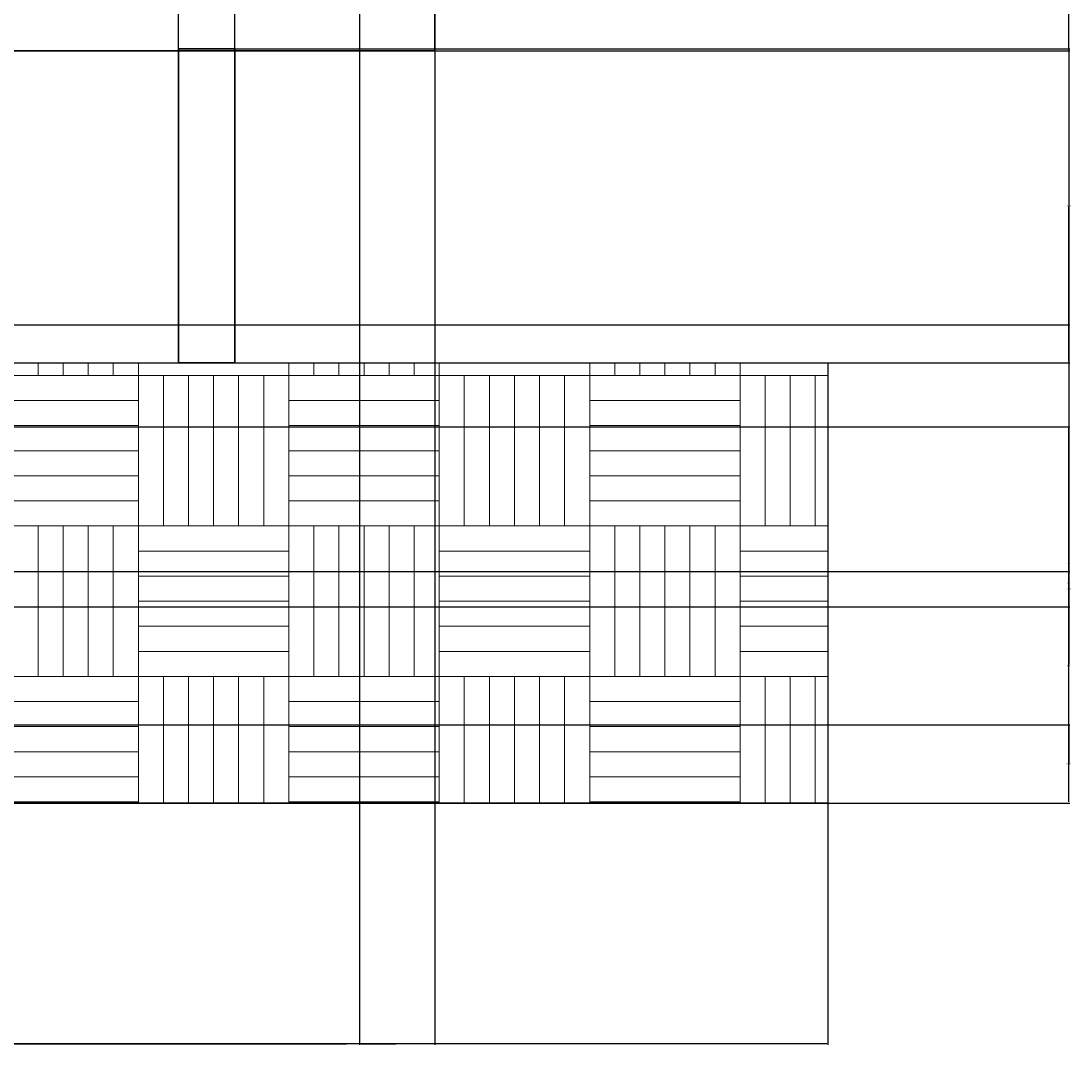
# Model space of a CAD drawing. Units: inches. Extents: x -15 to 605, y -220 to 570.
# Tile 5 of 10: x 438 to 605, y -155 to 9. Entities that reach past the tile are written whole.
import ezdxf

# ---------------------------------------------------------------- set-up
doc = ezdxf.new("R2010")
doc.units = ezdxf.units.IN
doc.header["$MEASUREMENT"] = 0
for name, color, linetype, lineweight in [('A-ANNO-DIMS', 2, 'Continuous', 18), ('A-COLS', 7, 'Continuous', 35), ('A-ELEV', 7, 'Continuous', 35), ('A-ELEV-PATT', 8, 'Continuous', 13), ('C-SITE', 3, 'Continuous', 25)]:
    doc.layers.add(name, color=color, linetype=linetype, lineweight=lineweight)
doc.styles.get("Standard").update_dxf_attribs({"font": 'arial.ttf'})
doc.dimstyles.get("Standard").update_dxf_attribs({"dimtxt": 0.18, "dimasz": 0.18, "dimexe": 0.18, "dimexo": 0.0625, "dimgap": 0.09, "dimtad": 0, "dimtih": 1, "dimtoh": 1, "dimdec": 4, "dimzin": 0, "dimdsep": 46, "dimtxsty": 'Standard', "dimcen": 0.09, "dimadec": 0, "dimazin": 0, "dimtfac": 1, "dimtdec": 4, "dimtofl": 0, "dimtmove": 0, "dimatfit": 3, "dimfxl": 1, "dimtolj": 1, "dimtzin": 0, "dimarcsym": 0})

# ---------------------------------------------------------------- blocks, each defined once
blk = doc.blocks.new('*D7')
at = {"layer": 'A-ANNO-DIMS', "color": 0, "lineweight": -2, "transparency": 16777216}
for p, q in [((23.99, 3.76), (23.99, -154.76)), ((566.72, -116.24), (566.72, -154.76)), ((24.17, -154.58), (294.96, -154.58)), ((566.54, -154.58), (295.75, -154.58))]:
    blk.add_line(p, q, dxfattribs=at)
at = {"layer": 'A-ANNO-DIMS', "color": 0, "transparency": 16777216}
for points in [[(24.17, -154.55), (24.17, -154.61), (23.99, -154.58)], [(566.54, -154.55), (566.54, -154.61), (566.72, -154.58)]]:
    blk.add_solid(points, dxfattribs=at)
at = {"layer": 'Defpoints', "color": 0, "transparency": 16777216}
for p in [(23.99, 3.82), (566.72, -116.18), (566.72, -154.58)]:
    blk.add_point(p, dxfattribs=at)
at = {"layer": 'A-ANNO-DIMS', "color": 0, "transparency": 16777216, "insert": (295.35, -154.58), "char_height": 0.18, "attachment_point": 5}
blk.add_mtext('\\A1;542.7', dxfattribs=at)
blk = doc.blocks.new('*D8')
at = {"layer": 'A-ANNO-DIMS', "color": 0, "lineweight": -2, "transparency": 16777216}
for p, q in [((23.99, 3.88), (23.99, 570.4)), ((24.17, 570.22), (263.7, 570.22)), ((503.81, 570.22), (264.28, 570.22)), ((503.99, 531.88), (503.99, 570.4))]:
    blk.add_line(p, q, dxfattribs=at)
at = {"layer": 'A-ANNO-DIMS', "color": 0, "transparency": 16777216}
for points in [[(24.17, 570.25), (24.17, 570.19), (23.99, 570.22)], [(503.81, 570.25), (503.81, 570.19), (503.99, 570.22)]]:
    blk.add_solid(points, dxfattribs=at)
at = {"layer": 'Defpoints', "color": 0, "transparency": 16777216}
for p in [(503.99, 570.22), (503.99, 531.82), (23.99, 3.82)]:
    blk.add_point(p, dxfattribs=at)
at = {"layer": 'A-ANNO-DIMS', "color": 0, "transparency": 16777216, "insert": (263.99, 570.22), "char_height": 0.18, "attachment_point": 5}
blk.add_mtext('\\A1;480', dxfattribs=at)
blk = doc.blocks.new('*D9')
at = {"layer": 'A-ANNO-DIMS', "color": 0, "lineweight": -2, "transparency": 16777216}
for p, q in [((503.92, 531.82), (-14.59, 531.82)), ((-14.41, 531.64), (-14.41, 208)), ((-14.41, -116), (-14.41, 207.64)), ((23.92, -116.18), (-14.59, -116.18))]:
    blk.add_line(p, q, dxfattribs=at)
at = {"layer": 'A-ANNO-DIMS', "color": 0, "transparency": 16777216}
for points in [[(-14.44, 531.64), (-14.38, 531.64), (-14.41, 531.82)], [(-14.44, -116), (-14.38, -116), (-14.41, -116.18)]]:
    blk.add_solid(points, dxfattribs=at)
at = {"layer": 'Defpoints', "color": 0, "transparency": 16777216}
for p in [(-14.41, 531.82), (503.99, 531.82), (23.99, -116.18)]:
    blk.add_point(p, dxfattribs=at)
at = {"layer": 'A-ANNO-DIMS', "color": 0, "transparency": 16777216, "insert": (-14.41, 207.82), "char_height": 0.18, "attachment_point": 5}
blk.add_mtext('\\A1;648', dxfattribs=at)
blk = doc.blocks.new('*D10')
at = {"layer": 'A-ANNO-DIMS', "color": 0, "lineweight": -2, "transparency": 16777216}
for p, q in [((504.05, 3.82), (605.3, 3.82)), ((605.12, 3.64), (605.12, -56)), ((605.12, -116), (605.12, -56.36)), ((566.78, -116.18), (605.3, -116.18))]:
    blk.add_line(p, q, dxfattribs=at)
at = {"layer": 'A-ANNO-DIMS', "color": 0, "transparency": 16777216}
for points in [[(605.09, 3.64), (605.15, 3.64), (605.12, 3.82)], [(605.09, -116), (605.15, -116), (605.12, -116.18)]]:
    blk.add_solid(points, dxfattribs=at)
at = {"layer": 'Defpoints', "color": 0, "transparency": 16777216}
for p in [(503.99, 3.82), (605.12, 3.82), (566.72, -116.18)]:
    blk.add_point(p, dxfattribs=at)
at = {"layer": 'A-ANNO-DIMS', "color": 0, "transparency": 16777216, "insert": (605.12, -56.18), "char_height": 0.18, "attachment_point": 5}
blk.add_mtext('\\A1;120', dxfattribs=at)
blk = doc.blocks.new('*D11')
at = {"layer": 'A-ANNO-DIMS', "color": 0, "lineweight": -2, "transparency": 16777216}
for p, q in [((492.05, 15.82), (605.3, 15.82)), ((605.12, 15.64), (605.12, 10)), ((605.12, 4), (605.12, 9.64)), ((504.05, 3.82), (605.3, 3.82))]:
    blk.add_line(p, q, dxfattribs=at)
at = {"layer": 'A-ANNO-DIMS', "color": 0, "transparency": 16777216}
for points in [[(605.09, 15.64), (605.15, 15.64), (605.12, 15.82)], [(605.09, 4), (605.15, 4), (605.12, 3.82)]]:
    blk.add_solid(points, dxfattribs=at)
at = {"layer": 'Defpoints', "color": 0, "transparency": 16777216}
for p in [(491.99, 15.82), (605.12, 15.82), (503.99, 3.82)]:
    blk.add_point(p, dxfattribs=at)
at = {"layer": 'A-ANNO-DIMS', "color": 0, "transparency": 16777216, "insert": (605.12, 9.82), "char_height": 0.18, "attachment_point": 5}
blk.add_mtext('\\A1;12', dxfattribs=at)
blk = doc.blocks.new('*D22')
at = {"layer": 'A-ANNO-DIMS', "color": 0, "lineweight": -2, "transparency": 16777216}
for p, q in [((472.17, 4.14), (605.3, 4.14)), ((605.12, 3.96), (605.12, -20.72)), ((605.12, -45.76), (605.12, -21.08)), ((472.17, -45.94), (605.3, -45.94))]:
    blk.add_line(p, q, dxfattribs=at)
at = {"layer": 'A-ANNO-DIMS', "color": 0, "transparency": 16777216}
for points in [[(605.09, 3.96), (605.15, 3.96), (605.12, 4.14)], [(605.09, -45.76), (605.15, -45.76), (605.12, -45.94)]]:
    blk.add_solid(points, dxfattribs=at)
at = {"layer": 'Defpoints', "color": 0, "transparency": 16777216}
for p in [(472.1, 4.14), (605.12, 4.14), (472.1, -45.94)]:
    blk.add_point(p, dxfattribs=at)
at = {"layer": 'A-ANNO-DIMS', "color": 0, "transparency": 16777216, "insert": (605.12, -20.9), "char_height": 0.18, "attachment_point": 5}
blk.add_mtext('\\A1;50.07', dxfattribs=at)
blk = doc.blocks.new('*D31')
at = {"layer": 'A-ANNO-DIMS', "color": 0, "lineweight": -2, "transparency": 16777216}
for p, q in [((382.03, 34.31), (382.03, -154.76)), ((491.99, 15.76), (491.99, -154.76)), ((382.21, -154.58), (436.55, -154.58)), ((491.81, -154.58), (437.46, -154.58))]:
    blk.add_line(p, q, dxfattribs=at)
at = {"layer": 'A-ANNO-DIMS', "color": 0, "transparency": 16777216}
for points in [[(382.21, -154.55), (382.21, -154.61), (382.03, -154.58)], [(491.81, -154.55), (491.81, -154.61), (491.99, -154.58)]]:
    blk.add_solid(points, dxfattribs=at)
at = {"layer": 'Defpoints', "color": 0, "transparency": 16777216}
for p in [(382.03, 34.38), (491.99, 15.82), (491.99, -154.58)]:
    blk.add_point(p, dxfattribs=at)
at = {"layer": 'A-ANNO-DIMS', "color": 0, "transparency": 16777216, "insert": (437.01, -154.58), "char_height": 0.18, "attachment_point": 5}
blk.add_mtext('\\A1;109.96', dxfattribs=at)
blk = doc.blocks.new('*D32')
at = {"layer": 'A-ANNO-DIMS', "color": 0, "lineweight": -2, "transparency": 16777216}
for p, q in [((491.99, 15.76), (491.99, -154.76)), ((503.99, 3.76), (503.99, -154.76)), ((492.17, -154.58), (497.78, -154.58)), ((503.81, -154.58), (498.2, -154.58))]:
    blk.add_line(p, q, dxfattribs=at)
at = {"layer": 'A-ANNO-DIMS', "color": 0, "transparency": 16777216}
for points in [[(492.17, -154.55), (492.17, -154.61), (491.99, -154.58)], [(503.81, -154.55), (503.81, -154.61), (503.99, -154.58)]]:
    blk.add_solid(points, dxfattribs=at)
at = {"layer": 'Defpoints', "color": 0, "transparency": 16777216}
for p in [(491.99, 15.82), (503.99, 3.82), (503.99, -154.58)]:
    blk.add_point(p, dxfattribs=at)
at = {"layer": 'A-ANNO-DIMS', "color": 0, "transparency": 16777216, "insert": (497.99, -154.58), "char_height": 0.18, "attachment_point": 5}
blk.add_mtext('\\A1;12', dxfattribs=at)
blk = doc.blocks.new('*D51')
at = {"layer": 'A-ANNO-DIMS', "color": 0, "lineweight": -2, "transparency": 16777216}
for p, q in [((414, -116.24), (414, -154.76)), ((566.72, -116.24), (566.72, -154.76)), ((414.18, -154.58), (489.9, -154.58)), ((566.54, -154.58), (490.81, -154.58))]:
    blk.add_line(p, q, dxfattribs=at)
at = {"layer": 'A-ANNO-DIMS', "color": 0, "transparency": 16777216}
for points in [[(414.18, -154.55), (414.18, -154.61), (414, -154.58)], [(566.54, -154.55), (566.54, -154.61), (566.72, -154.58)]]:
    blk.add_solid(points, dxfattribs=at)
at = {"layer": 'Defpoints', "color": 0, "transparency": 16777216}
for p in [(414, -116.18), (566.72, -116.18), (566.72, -154.58)]:
    blk.add_point(p, dxfattribs=at)
at = {"layer": 'A-ANNO-DIMS', "color": 0, "transparency": 16777216, "insert": (490.36, -154.58), "char_height": 0.18, "attachment_point": 5}
blk.add_mtext('\\A1;152.72', dxfattribs=at)
blk = doc.blocks.new('*D58')
at = {"layer": 'A-ANNO-DIMS', "color": 0, "lineweight": -2, "transparency": 16777216}
for p, q in [((376.71, -44.82), (376.71, 570.4)), ((376.89, 570.22), (419.58, 570.22)), ((462.92, 570.22), (420.23, 570.22)), ((463.1, -45.87), (463.1, 570.4))]:
    blk.add_line(p, q, dxfattribs=at)
at = {"layer": 'A-ANNO-DIMS', "color": 0, "transparency": 16777216}
for points in [[(376.89, 570.25), (376.89, 570.19), (376.71, 570.22)], [(462.92, 570.25), (462.92, 570.19), (463.1, 570.22)]]:
    blk.add_solid(points, dxfattribs=at)
at = {"layer": 'Defpoints', "color": 0, "transparency": 16777216}
for p in [(463.1, 570.22), (376.71, -44.88), (463.1, -45.94)]:
    blk.add_point(p, dxfattribs=at)
at = {"layer": 'A-ANNO-DIMS', "color": 0, "transparency": 16777216, "insert": (419.9, 570.22), "char_height": 0.18, "attachment_point": 5}
blk.add_mtext('\\A1;86.4', dxfattribs=at)
blk = doc.blocks.new('*D59')
at = {"layer": 'A-ANNO-DIMS', "color": 0, "lineweight": -2, "transparency": 16777216}
for p, q in [((463.1, -45.87), (463.1, 570.4)), ((463.28, 570.22), (467.45, 570.22)), ((471.92, 570.22), (467.75, 570.22)), ((472.1, -45.87), (472.1, 570.4))]:
    blk.add_line(p, q, dxfattribs=at)
at = {"layer": 'A-ANNO-DIMS', "color": 0, "transparency": 16777216}
for points in [[(463.28, 570.25), (463.28, 570.19), (463.1, 570.22)], [(471.92, 570.25), (471.92, 570.19), (472.1, 570.22)]]:
    blk.add_solid(points, dxfattribs=at)
at = {"layer": 'Defpoints', "color": 0, "transparency": 16777216}
for p in [(472.1, 570.22), (463.1, -45.94), (472.1, -45.94)]:
    blk.add_point(p, dxfattribs=at)
at = {"layer": 'A-ANNO-DIMS', "color": 0, "transparency": 16777216, "insert": (467.6, 570.22), "char_height": 0.18, "attachment_point": 5}
blk.add_mtext('\\A1;9', dxfattribs=at)
blk = doc.blocks.new('*D63')
at = {"layer": 'A-ANNO-DIMS', "color": 0, "lineweight": -2, "transparency": 16777216}
for p, q in [((392.68, -39.88), (605.3, -39.88)), ((605.12, -40.06), (605.12, -77.85)), ((605.12, -116), (605.12, -78.21)), ((370.91, -116.18), (605.3, -116.18))]:
    blk.add_line(p, q, dxfattribs=at)
at = {"layer": 'A-ANNO-DIMS', "color": 0, "transparency": 16777216}
for points in [[(605.09, -40.06), (605.15, -40.06), (605.12, -39.88)], [(605.09, -116), (605.15, -116), (605.12, -116.18)]]:
    blk.add_solid(points, dxfattribs=at)
at = {"layer": 'Defpoints', "color": 0, "transparency": 16777216}
for p in [(392.61, -39.88), (605.12, -39.88), (370.85, -116.18)]:
    blk.add_point(p, dxfattribs=at)
at = {"layer": 'A-ANNO-DIMS', "color": 0, "transparency": 16777216, "insert": (605.12, -78.03), "char_height": 0.18, "attachment_point": 5}
blk.add_mtext('\\A1;76.3', dxfattribs=at)
blk = doc.blocks.new('*D67')
at = {"layer": 'A-ANNO-DIMS', "color": 0, "lineweight": -2, "transparency": 16777216}
for p, q in [((566.78, -45.94), (605.3, -45.94)), ((605.12, -46.12), (605.12, -80.88)), ((605.12, -116), (605.12, -81.24)), ((566.78, -116.18), (605.3, -116.18))]:
    blk.add_line(p, q, dxfattribs=at)
at = {"layer": 'A-ANNO-DIMS', "color": 0, "transparency": 16777216}
for points in [[(605.09, -46.12), (605.15, -46.12), (605.12, -45.94)], [(605.09, -116), (605.15, -116), (605.12, -116.18)]]:
    blk.add_solid(points, dxfattribs=at)
at = {"layer": 'Defpoints', "color": 0, "transparency": 16777216}
for p in [(566.72, -45.94), (605.12, -45.94), (566.72, -116.18)]:
    blk.add_point(p, dxfattribs=at)
at = {"layer": 'A-ANNO-DIMS', "color": 0, "transparency": 16777216, "insert": (605.12, -81.06), "char_height": 0.18, "attachment_point": 5}
blk.add_mtext('\\A1;70.24', dxfattribs=at)
blk = doc.blocks.new('*D68')
at = {"layer": 'A-ANNO-DIMS', "color": 0, "lineweight": -2, "transparency": 16777216}
for p, q in [((252.05, -56.18), (605.3, -56.18)), ((605.12, -56.36), (605.12, -86)), ((605.12, -116), (605.12, -86.36)), ((252.05, -116.18), (605.3, -116.18))]:
    blk.add_line(p, q, dxfattribs=at)
at = {"layer": 'A-ANNO-DIMS', "color": 0, "transparency": 16777216}
for points in [[(605.09, -56.36), (605.15, -56.36), (605.12, -56.18)], [(605.09, -116), (605.15, -116), (605.12, -116.18)]]:
    blk.add_solid(points, dxfattribs=at)
at = {"layer": 'Defpoints', "color": 0, "transparency": 16777216}
for p in [(251.99, -56.18), (605.12, -56.18), (251.99, -116.18)]:
    blk.add_point(p, dxfattribs=at)
at = {"layer": 'A-ANNO-DIMS', "color": 0, "transparency": 16777216, "insert": (605.12, -86.18), "char_height": 0.18, "attachment_point": 5}
blk.add_mtext('\\A1;60', dxfattribs=at)
blk = doc.blocks.new('*D107')
at = {"layer": 'A-ANNO-DIMS', "color": 0, "lineweight": -2, "transparency": 16777216}
for p, q in [((303.23, -103.68), (605.3, -103.68)), ((605.12, -103.86), (605.12, -109.75)), ((605.12, -116), (605.12, -110.11)), ((330.5, -116.18), (605.3, -116.18))]:
    blk.add_line(p, q, dxfattribs=at)
at = {"layer": 'A-ANNO-DIMS', "color": 0, "transparency": 16777216}
for points in [[(605.09, -103.86), (605.15, -103.86), (605.12, -103.68)], [(605.09, -116), (605.15, -116), (605.12, -116.18)]]:
    blk.add_solid(points, dxfattribs=at)
at = {"layer": 'Defpoints', "color": 0, "transparency": 16777216}
for p in [(303.17, -103.68), (605.12, -103.68), (330.43, -116.18)]:
    blk.add_point(p, dxfattribs=at)
at = {"layer": 'A-ANNO-DIMS', "color": 0, "transparency": 16777216, "insert": (605.12, -109.93), "char_height": 0.18, "attachment_point": 5}
blk.add_mtext('\\A1;12.503', dxfattribs=at)
blk = doc.blocks.new('*D108')
at = {"layer": 'A-ANNO-DIMS', "color": 0, "lineweight": -2, "transparency": 16777216}
for p, q in [((283.65, -84.86), (605.3, -84.86)), ((605.12, -85.04), (605.12, -94.09)), ((605.12, -103.5), (605.12, -94.45)), ((303.23, -103.68), (605.3, -103.68))]:
    blk.add_line(p, q, dxfattribs=at)
at = {"layer": 'A-ANNO-DIMS', "color": 0, "transparency": 16777216}
for points in [[(605.09, -85.04), (605.15, -85.04), (605.12, -84.86)], [(605.09, -103.5), (605.15, -103.5), (605.12, -103.68)]]:
    blk.add_solid(points, dxfattribs=at)
at = {"layer": 'Defpoints', "color": 0, "transparency": 16777216}
for p in [(283.59, -84.86), (605.12, -84.86), (303.17, -103.68)]:
    blk.add_point(p, dxfattribs=at)
at = {"layer": 'A-ANNO-DIMS', "color": 0, "transparency": 16777216, "insert": (605.12, -94.27), "char_height": 0.18, "attachment_point": 5}
blk.add_mtext('\\A1;18.82', dxfattribs=at)
blk = doc.blocks.new('*D109')
at = {"layer": 'A-ANNO-DIMS', "color": 0, "lineweight": -2, "transparency": 16777216}
for p, q in [((308.92, -79.22), (605.3, -79.22)), ((605.12, -79.4), (605.12, -81.86)), ((605.12, -84.68), (605.12, -82.22)), ((283.65, -84.86), (605.3, -84.86))]:
    blk.add_line(p, q, dxfattribs=at)
at = {"layer": 'A-ANNO-DIMS', "color": 0, "transparency": 16777216}
for points in [[(605.09, -79.4), (605.15, -79.4), (605.12, -79.22)], [(605.09, -84.68), (605.15, -84.68), (605.12, -84.86)]]:
    blk.add_solid(points, dxfattribs=at)
at = {"layer": 'Defpoints', "color": 0, "transparency": 16777216}
for p in [(308.86, -79.22), (605.12, -79.22), (283.59, -84.86)]:
    blk.add_point(p, dxfattribs=at)
at = {"layer": 'A-ANNO-DIMS', "color": 0, "transparency": 16777216, "insert": (605.12, -82.04), "char_height": 0.18, "attachment_point": 5}
blk.add_mtext('\\A1;5.637', dxfattribs=at)

msp = doc.modelspace()

# ---------------------------------------------------------------- hatches: boundary and pattern name
at = {"layer": 'A-ELEV-PATT'}
h = msp.add_hatch(dxfattribs=at)
h.set_pattern_fill('AR-PARQ1', color=256, scale=2)
h.set_pattern_definition([(90, (-191.319, 0), (-24, 24), [24, -24]), (90, (-187.319, 0), (-24, 24), [24, -24]), (90, (-183.319, 0), (-24, 24), [24, -24]), (90, (-179.319, 0), (-24, 24), [24, -24]), (90, (-175.319, 0), (-24, 24), [24, -24]), (90, (-171.319, 0), (-24, 24), [24, -24]), (90, (-167.319, 0), (-24, 24), [24, -24]), (0, (-191.319, 24), (24, -24), [24, -24]), (0, (-191.319, 28), (24, -24), [24, -24]), (0, (-191.319, 32), (24, -24), [24, -24]), (0, (-191.319, 36), (24, -24), [24, -24]), (0, (-191.319, 40), (24, -24), [24, -24]), (0, (-191.319, 44), (24, -24), [24, -24]), (0, (-191.319, 48), (24, -24), [24, -24])])
h.paths.add_polyline_path([(392.6125, -39.8843), (378.2334, -39.8843), (354.916, -116.1813), (370.8496, -116.1813)])
h.paths.add_polyline_path([(368.1292, -39.8843), (353.7501, -39.8843), (330.4327, -116.1813), (346.3663, -116.1813)])
h.paths.add_polyline_path([(566.7161, -45.9373), (413.9976, -45.9373), (413.9976, -116.1813), (566.7161, -116.1813)])
h.paths.add_polyline_path([(251.9872, -35.1813), (227.9872, -35.1813), (227.9872, -116.1813), (251.9872, -116.1813)])
h.paths.add_polyline_path([(83.9872, -35.1813), (23.9872, -35.1813), (23.9872, -116.1813), (83.9872, -116.1813), (83.9872, -113.1422)])
h.paths.add_polyline_path([(72.6838, -44.8238), (72.6838, -109.4483), (32.7886, -109.4483), (32.7886, -44.8238)], flags=16)

# ---------------------------------------------------------------- linework, layer by layer
at = {"layer": 'A-COLS'}
msp.add_lwpolyline([(463.1032, -45.9373), (472.1032, -45.9373), (472.1032, 4.1352), (463.1032, 4.1352)], close=True, dxfattribs=at)
at = {"layer": 'A-ELEV'}
msp.add_lwpolyline([(23.9872, 123.8187), (23.9872, 3.8187), (503.9872, 3.8187), (503.9872, 123.8187), (503.9872, 531.8187)], dxfattribs=at)
at = {"layer": 'C-SITE'}
msp.add_line((23.9872, -116.1813), (503.9872, -116.1813), dxfattribs=at)
msp.add_lwpolyline([(413.9976, -45.9373), (566.7161, -45.9373), (566.7161, -116.1813), (413.9976, -116.1813)], close=True, dxfattribs=at)

# ---------------------------------------------------------------- dimensions: what is measured, and where the dimension line sits
at = {"layer": 'A-ANNO-DIMS'}
for base, p1, p2, override, picture, middle in [((503.9872, 570.2187), (23.9872, 3.8187), (503.9872, 531.8187), {"dimdec": 0, "dimlfac": 1, "dimrnd": 0, "dimzin": 0, "dimdsep": 46, "dimlunit": 2}, '*D8', (263.9872, 570.2187)), ((463.1032, 570.2187), (376.7066, -44.8803), (463.1032, -45.9373), {"dimdec": 1, "dimlfac": 1, "dimrnd": 0, "dimzin": 0, "dimdsep": 46, "dimlunit": 2}, '*D58', (419.9049, 570.2187)), ((472.1032, 570.2187), (463.1032, -45.9373), (472.1032, -45.9373), {"dimdec": 0, "dimlfac": 1, "dimrnd": 0, "dimzin": 0, "dimdsep": 46, "dimlunit": 2}, '*D59', (467.6032, 570.2187)), ((491.9872, -154.5813), (382.0304, 34.3758), (491.9872, 15.8187), {"dimdec": 2, "dimlfac": 1, "dimrnd": 0, "dimzin": 0, "dimdsep": 46, "dimlunit": 2}, '*D31', (437.0088, -154.5813)), ((503.9872, -154.5813), (491.9872, 15.8187), (503.9872, 3.8187), {"dimdec": 0, "dimlfac": 1, "dimrnd": 0, "dimzin": 0, "dimdsep": 46, "dimlunit": 2}, '*D32', (497.9872, -154.5813)), ((566.7161, -154.5813), (23.9872, 3.8187), (566.7161, -116.1813), {"dimdec": 1, "dimlfac": 1, "dimrnd": 0, "dimzin": 0, "dimdsep": 46, "dimlunit": 2}, '*D7', (295.3517, -154.5813)), ((566.7161, -154.5813), (413.9976, -116.1813), (566.7161, -116.1813), {"dimdec": 2, "dimlfac": 1, "dimrnd": 0, "dimzin": 0, "dimdsep": 46, "dimlunit": 2}, '*D51', (490.3568, -154.5813))]:
    dim = msp.add_linear_dim(base=base, p1=p1, p2=p2, dimstyle='Standard', override=override, dxfattribs=at)
    dim.commit()
    dim.dimension.update_dxf_attribs({"geometry": picture, "text_midpoint": middle})
for base, p1, p2, override, picture, middle in [((-14.4128, 531.8187), (23.9872, -116.1813), (503.9872, 531.8187), {"dimdec": 0, "dimlfac": 1, "dimrnd": 0, "dimzin": 0, "dimdsep": 46, "dimlunit": 2}, '*D9', (-14.4128, 207.8187)), ((605.1161, 15.8187), (503.9872, 3.8187), (491.9872, 15.8187), {"dimdec": 0, "dimlfac": 1, "dimrnd": 0, "dimzin": 0, "dimdsep": 46, "dimlunit": 2}, '*D11', (605.1161, 9.8187)), ((605.1161, 4.1352), (472.1032, -45.9373), (472.1032, 4.1352), {"dimdec": 2, "dimlfac": 1, "dimrnd": 0, "dimzin": 0, "dimdsep": 46, "dimlunit": 2}, '*D22', (605.1161, -20.9011)), ((605.1161, 3.8187), (566.7161, -116.1813), (503.9872, 3.8187), {"dimdec": 0, "dimlfac": 1, "dimrnd": 0, "dimzin": 0, "dimdsep": 46, "dimlunit": 2}, '*D10', (605.1161, -56.1813)), ((605.1161, -39.8843), (370.8496, -116.1813), (392.6125, -39.8843), {"dimdec": 1, "dimlfac": 1, "dimrnd": 0, "dimzin": 0, "dimdsep": 46, "dimlunit": 2}, '*D63', (605.1161, -78.0328)), ((605.1161, -45.9373), (566.7161, -116.1813), (566.7161, -45.9373), {"dimdec": 2, "dimlfac": 1, "dimrnd": 0, "dimzin": 0, "dimdsep": 46, "dimlunit": 2}, '*D67', (605.1161, -81.0593)), ((605.1161, -56.1813), (251.9872, -116.1813), (251.9872, -56.1813), {"dimdec": 0, "dimlfac": 1, "dimrnd": 0, "dimzin": 0, "dimdsep": 46, "dimlunit": 2}, '*D68', (605.1161, -86.1813)), ((605.1161, -79.2202), (283.5871, -84.8572), (308.8611, -79.2202), {"dimdec": 3, "dimlfac": 1, "dimrnd": 0, "dimzin": 0, "dimdsep": 46, "dimlunit": 2}, '*D109', (605.1161, -82.0387)), ((605.1161, -84.8572), (303.1719, -103.6786), (283.5871, -84.8572), {"dimdec": 2, "dimlfac": 1, "dimrnd": 0, "dimzin": 0, "dimdsep": 46, "dimlunit": 2}, '*D108', (605.1161, -94.2679)), ((605.1161, -103.6786), (330.4327, -116.1813), (303.1719, -103.6786), {"dimdec": 3, "dimlfac": 1, "dimrnd": 0, "dimzin": 0, "dimdsep": 46, "dimlunit": 2}, '*D107', (605.1161, -109.9299))]:
    dim = msp.add_linear_dim(base=base, p1=p1, p2=p2, angle=90, dimstyle='Standard', override=override, dxfattribs=at)
    dim.commit()
    dim.dimension.update_dxf_attribs({"geometry": picture, "text_midpoint": middle})

doc.saveas('drawing.dxf')
